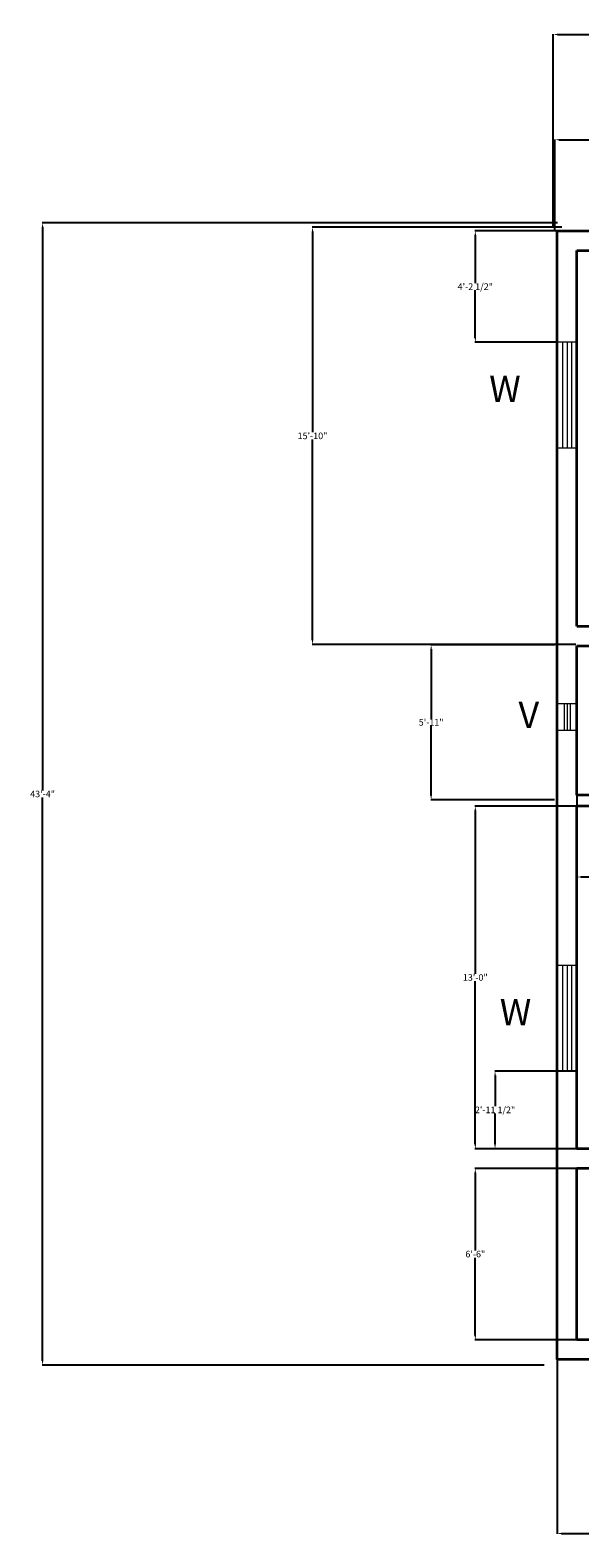
# Model space of a CAD drawing. Units: inches. Extents: x 751 to 1500, y 610 to 1297.
# Tile 1 of 4: x 751 to 1001, y 610 to 1297. Entities that reach past the tile are written whole.
import ezdxf

# ---------------------------------------------------------------- set-up
doc = ezdxf.new("R2010")
doc.units = ezdxf.units.IN
doc.header["$MEASUREMENT"] = 0
doc.layers.get('0').update_dxf_attribs({"color": 1})
for name, color, linetype, lineweight in [('A-ANNO-DIMS', 5, 'Continuous', 18), ('A-ANNO-TEXT', 7, 'Continuous', 18), ('wall', 6, 'Continuous', 35), ('windows', 70, 'Continuous', 18)]:
    doc.layers.add(name, color=color, linetype=linetype, lineweight=lineweight)
doc.styles.get("Standard").update_dxf_attribs({"font": 'arial.ttf'})
doc.dimstyles.get("Standard").update_dxf_attribs({"dimtxt": 3, "dimasz": 2, "dimexe": 0.18, "dimexo": 0.0625, "dimgap": 0.09, "dimtad": 0, "dimtih": 1, "dimtoh": 1, "dimdec": 0, "dimzin": 0, "dimdsep": 46, "dimlunit": 3, "dimtxsty": 'Standard', "dimcen": 0.09, "dimadec": 0, "dimazin": 0, "dimtfac": 1, "dimtdec": 0, "dimtofl": 0, "dimtmove": 0, "dimatfit": 3, "dimfxl": 1, "dimtolj": 1, "dimtzin": 0, "dimarcsym": 0})

# ---------------------------------------------------------------- blocks, each defined once
blk = doc.blocks.new('*D8')
at = {"layer": 'A-ANNO-DIMS', "color": 0, "lineweight": -2, "transparency": 16777216}
for p, q in [((989.16, 1207.18), (989.16, 1295.32)), ((991.16, 1295.14), (1215.8, 1295.14)), ((1450.93, 1295.14), (1226.29, 1295.14)), ((1452.93, 1205.96), (1452.93, 1295.32))]:
    blk.add_line(p, q, dxfattribs=at)
at = {"layer": 'A-ANNO-DIMS', "color": 0, "transparency": 16777216}
for points in [[(991.16, 1295.48), (991.16, 1294.81), (989.16, 1295.14)], [(1450.93, 1295.48), (1450.93, 1294.81), (1452.93, 1295.14)]]:
    blk.add_solid(points, dxfattribs=at)
at = {"layer": 'Defpoints', "color": 0, "transparency": 16777216}
for p in [(1452.93, 1295.14), (989.16, 1207.12), (1452.93, 1205.9)]:
    blk.add_point(p, dxfattribs=at)
at = {"layer": 'A-ANNO-DIMS', "color": 0, "transparency": 16777216, "insert": (1221.05, 1295.14), "char_height": 3, "attachment_point": 5}
blk.add_mtext('\\A1;38\'-8"', dxfattribs=at)
blk = doc.blocks.new('*D9')
at = {"layer": 'A-ANNO-DIMS', "color": 0, "lineweight": -2, "transparency": 16777216}
for p, q in [((989.97, 1205.95), (989.97, 1247.37)), ((991.97, 1247.19), (1077.79, 1247.19)), ((1173.82, 1247.19), (1088, 1247.19)), ((1175.82, 1205.95), (1175.82, 1247.37))]:
    blk.add_line(p, q, dxfattribs=at)
at = {"layer": 'A-ANNO-DIMS', "color": 0, "transparency": 16777216}
for points in [[(991.97, 1247.53), (991.97, 1246.86), (989.97, 1247.19)], [(1173.82, 1247.53), (1173.82, 1246.86), (1175.82, 1247.19)]]:
    blk.add_solid(points, dxfattribs=at)
at = {"layer": 'Defpoints', "color": 0, "transparency": 16777216}
for p in [(1175.82, 1247.19), (989.97, 1205.88), (1175.82, 1205.88)]:
    blk.add_point(p, dxfattribs=at)
at = {"layer": 'A-ANNO-DIMS', "color": 0, "transparency": 16777216, "insert": (1082.89, 1247.19), "char_height": 3, "attachment_point": 5}
blk.add_mtext('\\A1;15\'-6"', dxfattribs=at)
blk = doc.blocks.new('*D12')
at = {"layer": 'A-ANNO-DIMS', "color": 0, "lineweight": -2, "transparency": 16777216}
for p, q in [((991.09, 1209.39), (756.58, 1209.39)), ((756.76, 1207.39), (756.76, 950.89)), ((756.76, 691.14), (756.76, 947.64)), ((985.08, 689.14), (756.58, 689.14))]:
    blk.add_line(p, q, dxfattribs=at)
at = {"layer": 'A-ANNO-DIMS', "color": 0, "transparency": 16777216}
for points in [[(756.42, 1207.39), (757.09, 1207.39), (756.76, 1209.39)], [(756.42, 691.14), (757.09, 691.14), (756.76, 689.14)]]:
    blk.add_solid(points, dxfattribs=at)
at = {"layer": 'Defpoints', "color": 0, "transparency": 16777216}
for p in [(991.15, 1209.39), (756.76, 689.14), (985.14, 689.14)]:
    blk.add_point(p, dxfattribs=at)
at = {"layer": 'A-ANNO-DIMS', "color": 0, "transparency": 16777216, "insert": (756.76, 949.26), "char_height": 3, "attachment_point": 5}
blk.add_mtext('\\A1;43\'-4"', dxfattribs=at)
blk = doc.blocks.new('*D13')
at = {"layer": 'A-ANNO-DIMS', "color": 0, "lineweight": -2, "transparency": 16777216}
for p, q in [((993.09, 1207.39), (879.45, 1207.39)), ((879.63, 1205.39), (879.63, 1113.96)), ((879.63, 1019.29), (879.63, 1110.72)), ((999.43, 1017.29), (879.45, 1017.29))]:
    blk.add_line(p, q, dxfattribs=at)
at = {"layer": 'A-ANNO-DIMS', "color": 0, "transparency": 16777216}
for points in [[(879.3, 1205.39), (879.97, 1205.39), (879.63, 1207.39)], [(879.3, 1019.29), (879.97, 1019.29), (879.63, 1017.29)]]:
    blk.add_solid(points, dxfattribs=at)
at = {"layer": 'Defpoints', "color": 0, "transparency": 16777216}
for p in [(993.15, 1207.39), (879.63, 1017.29), (999.5, 1017.29)]:
    blk.add_point(p, dxfattribs=at)
at = {"layer": 'A-ANNO-DIMS', "color": 0, "transparency": 16777216, "insert": (879.63, 1112.34), "char_height": 3, "attachment_point": 5}
blk.add_mtext('\\A1;15\'-10"', dxfattribs=at)
blk = doc.blocks.new('*D14')
at = {"layer": 'A-ANNO-DIMS', "color": 0, "lineweight": -2, "transparency": 16777216}
for p, q in [((989.87, 1017.15), (933.44, 1017.15)), ((933.62, 1015.15), (933.62, 983.5)), ((933.62, 948.6), (933.62, 980.25)), ((989.8, 946.6), (933.44, 946.6))]:
    blk.add_line(p, q, dxfattribs=at)
at = {"layer": 'A-ANNO-DIMS', "color": 0, "transparency": 16777216}
for points in [[(933.29, 1015.15), (933.96, 1015.15), (933.62, 1017.15)], [(933.29, 948.6), (933.96, 948.6), (933.62, 946.6)]]:
    blk.add_solid(points, dxfattribs=at)
at = {"layer": 'Defpoints', "color": 0, "transparency": 16777216}
for p in [(989.93, 1017.15), (933.62, 946.6), (989.86, 946.6)]:
    blk.add_point(p, dxfattribs=at)
at = {"layer": 'A-ANNO-DIMS', "color": 0, "transparency": 16777216, "insert": (933.62, 981.87), "char_height": 3, "attachment_point": 5}
blk.add_mtext('\\A1;5\'-11"', dxfattribs=at)
blk = doc.blocks.new('WIN-48IN-PLAN')
for p, q in [((2.5, 48), (2.5, 0)), ((4.5, 48), (4.5, 0)), ((6.5, 48), (6.5, 0))]:
    blk.add_line(p, q)
blk.add_lwpolyline([(9, 48), (0, 48), (0, 0), (9, 0)], close=True)
blk = doc.blocks.new('VENT-12IN-PLAN')
for p, q in [((3.14, 12), (3.14, 0)), ((4.5, 12), (4.5, 0)), ((5.86, 12), (5.86, 0))]:
    blk.add_line(p, q)
blk.add_lwpolyline([(0, 0), (9, 0), (9, 12), (0, 12)], close=True)
blk = doc.blocks.new('*D47')
at = {"layer": 'A-ANNO-DIMS', "color": 0, "lineweight": -2, "transparency": 16777216}
for p, q in [((990.98, 691.63), (990.98, 612.26)), ((1176.98, 691.63), (1176.98, 612.26)), ((992.98, 612.44), (1078.88, 612.44)), ((1174.98, 612.44), (1089.08, 612.44))]:
    blk.add_line(p, q, dxfattribs=at)
at = {"layer": 'A-ANNO-DIMS', "color": 0, "transparency": 16777216}
for points in [[(992.98, 612.77), (992.98, 612.11), (990.98, 612.44)], [(1174.98, 612.77), (1174.98, 612.11), (1176.98, 612.44)]]:
    blk.add_solid(points, dxfattribs=at)
at = {"layer": 'Defpoints', "color": 0, "transparency": 16777216}
for p in [(990.98, 691.69), (1176.98, 691.69), (1176.98, 612.44)]:
    blk.add_point(p, dxfattribs=at)
at = {"layer": 'A-ANNO-DIMS', "color": 0, "transparency": 16777216, "insert": (1083.98, 612.44), "char_height": 3, "attachment_point": 5}
blk.add_mtext('\\A1;15\'-6"', dxfattribs=at)
blk = doc.blocks.new('*D49')
at = {"layer": 'A-ANNO-DIMS', "color": 0, "lineweight": -2, "transparency": 16777216}
for p, q in [((999.92, 778.69), (953.55, 778.69)), ((953.73, 776.69), (953.73, 741.31)), ((953.73, 702.69), (953.73, 738.07)), ((999.92, 700.69), (953.55, 700.69))]:
    blk.add_line(p, q, dxfattribs=at)
at = {"layer": 'A-ANNO-DIMS', "color": 0, "transparency": 16777216}
for points in [[(953.4, 776.69), (954.07, 776.69), (953.73, 778.69)], [(953.4, 702.69), (954.07, 702.69), (953.73, 700.69)]]:
    blk.add_solid(points, dxfattribs=at)
at = {"layer": 'Defpoints', "color": 0, "transparency": 16777216}
for p in [(953.73, 778.69), (999.98, 778.69), (999.98, 700.69)]:
    blk.add_point(p, dxfattribs=at)
at = {"layer": 'A-ANNO-DIMS', "color": 0, "transparency": 16777216, "insert": (953.73, 739.69), "char_height": 3, "attachment_point": 5}
blk.add_mtext('\\A1;6\'-6"', dxfattribs=at)
blk = doc.blocks.new('*D50')
at = {"layer": 'A-ANNO-DIMS', "color": 0, "lineweight": -2, "transparency": 16777216}
for p, q in [((999.92, 943.69), (953.55, 943.69)), ((953.73, 941.69), (953.73, 867.31)), ((953.73, 789.69), (953.73, 864.07)), ((999.92, 787.69), (953.55, 787.69))]:
    blk.add_line(p, q, dxfattribs=at)
at = {"layer": 'A-ANNO-DIMS', "color": 0, "transparency": 16777216}
for points in [[(953.4, 941.69), (954.07, 941.69), (953.73, 943.69)], [(953.4, 789.69), (954.07, 789.69), (953.73, 787.69)]]:
    blk.add_solid(points, dxfattribs=at)
at = {"layer": 'Defpoints', "color": 0, "transparency": 16777216}
for p in [(953.73, 943.69), (999.98, 943.69), (999.98, 787.69)]:
    blk.add_point(p, dxfattribs=at)
at = {"layer": 'A-ANNO-DIMS', "color": 0, "transparency": 16777216, "insert": (953.73, 865.69), "char_height": 3, "attachment_point": 5}
blk.add_mtext('\\A1;13\'-0"', dxfattribs=at)
blk = doc.blocks.new('*D54')
at = {"layer": 'A-ANNO-DIMS', "color": 0, "lineweight": -2, "transparency": 16777216}
for p, q in [((999.98, 948.63), (999.98, 911.26)), ((1083.98, 948.63), (1083.98, 911.26)), ((1001.98, 911.44), (1037.92, 911.44)), ((1081.98, 911.44), (1046.05, 911.44))]:
    blk.add_line(p, q, dxfattribs=at)
at = {"layer": 'A-ANNO-DIMS', "color": 0, "transparency": 16777216}
for points in [[(1001.98, 911.77), (1001.98, 911.11), (999.98, 911.44)], [(1081.98, 911.77), (1081.98, 911.11), (1083.98, 911.44)]]:
    blk.add_solid(points, dxfattribs=at)
at = {"layer": 'Defpoints', "color": 0, "transparency": 16777216}
for p in [(999.98, 948.69), (1083.98, 948.69), (999.98, 911.44)]:
    blk.add_point(p, dxfattribs=at)
at = {"layer": 'A-ANNO-DIMS', "color": 0, "transparency": 16777216, "insert": (1041.98, 911.44), "char_height": 3, "attachment_point": 5}
blk.add_mtext('\\A1;7\'-0"', dxfattribs=at)
blk = doc.blocks.new('*D63')
at = {"layer": 'A-ANNO-DIMS', "color": 0, "lineweight": -2, "transparency": 16777216}
for p, q in [((990.92, 1205.69), (953.55, 1205.69)), ((953.73, 1203.69), (953.73, 1181.96)), ((953.73, 1156.94), (953.73, 1178.68)), ((990.92, 1154.94), (953.55, 1154.94))]:
    blk.add_line(p, q, dxfattribs=at)
at = {"layer": 'A-ANNO-DIMS', "color": 0, "transparency": 16777216}
for points in [[(953.4, 1203.69), (954.07, 1203.69), (953.73, 1205.69)], [(953.4, 1156.94), (954.07, 1156.94), (953.73, 1154.94)]]:
    blk.add_solid(points, dxfattribs=at)
at = {"layer": 'Defpoints', "color": 0, "transparency": 16777216}
for p in [(953.73, 1205.69), (990.98, 1205.69), (990.98, 1154.94)]:
    blk.add_point(p, dxfattribs=at)
at = {"layer": 'A-ANNO-DIMS', "color": 0, "transparency": 16777216, "insert": (953.73, 1180.32), "char_height": 3, "attachment_point": 5}
blk.add_mtext('\\A1;4\'-2 1/2"', dxfattribs=at)
blk = doc.blocks.new('*D64')
at = {"layer": 'A-ANNO-DIMS', "color": 0, "lineweight": -2, "transparency": 16777216}
for p, q in [((999.92, 823.06), (962.55, 823.06)), ((962.73, 821.06), (962.73, 807.02)), ((962.73, 789.69), (962.73, 803.74)), ((999.92, 787.69), (962.55, 787.69))]:
    blk.add_line(p, q, dxfattribs=at)
at = {"layer": 'A-ANNO-DIMS', "color": 0, "transparency": 16777216}
for points in [[(962.4, 821.06), (963.07, 821.06), (962.73, 823.06)], [(962.4, 789.69), (963.07, 789.69), (962.73, 787.69)]]:
    blk.add_solid(points, dxfattribs=at)
at = {"layer": 'Defpoints', "color": 0, "transparency": 16777216}
for p in [(962.73, 823.06), (999.98, 823.06), (999.98, 787.69)]:
    blk.add_point(p, dxfattribs=at)
at = {"layer": 'A-ANNO-DIMS', "color": 0, "transparency": 16777216, "insert": (962.73, 805.38), "char_height": 3, "attachment_point": 5}
blk.add_mtext('\\A1;2\'-11 1/2"', dxfattribs=at)

msp = doc.modelspace()

# ---------------------------------------------------------------- linework, layer by layer
at = {"layer": 'wall'}
for p, q in [((990.98, 986.69), (990.98, 1205.69)), ((990.98, 1205.69), (1296.98, 1205.69)), ((999.98, 1196.69), (1171.98, 1196.69)), ((999.98, 1025.69), (999.98, 1196.69)), ((999.98, 1025.69), (1054.98, 1025.69)), ((999.98, 986.69), (999.98, 1016.69)), ((999.98, 1016.69), (1054.98, 1016.69)), ((990.98, 932.69), (990.98, 986.69)), ((999.98, 948.69), (999.98, 986.69)), ((1083.98, 948.69), (999.98, 948.69)), ((999.98, 932.69), (999.98, 943.69)), ((1171.98, 943.69), (999.98, 943.69)), ((990.98, 760.69), (990.98, 932.69)), ((999.98, 787.69), (999.98, 932.69)), ((1182.32, 787.69), (999.98, 787.69)), ((999.98, 760.69), (999.98, 778.69)), ((999.98, 700.69), (999.98, 778.69)), ((1182.32, 778.69), (999.98, 778.69)), ((990.98, 691.69), (990.98, 760.69)), ((1306.98, 700.69), (999.98, 700.69)), ((1171.98, 691.69), (990.98, 691.69))]:
    msp.add_line(p, q, dxfattribs=at)
at = {"layer": 'windows'}
for p, q in [((997.48, 871.06), (997.48, 823.06)), ((999.98, 871.06), (999.98, 823.06))]:
    msp.add_line(p, q, dxfattribs=at)
msp.add_lwpolyline([(999.98, 871.06), (990.98, 871.06), (990.98, 823.06), (999.98, 823.06)], close=True, dxfattribs=at)

# ---------------------------------------------------------------- block references
for name, p in [('WIN-48IN-PLAN', (990.98, 1106.94)), ('WIN-48IN-PLAN', (990.98, 1106.94)), ('VENT-12IN-PLAN', (990.98, 978.34)), ('WIN-48IN-PLAN', (990.98, 823.06))]:
    msp.add_blockref(name, p, dxfattribs=at)

# ---------------------------------------------------------------- texts
at = {"layer": 'A-ANNO-TEXT', "char_height": 12, "attachment_point": 1}
for s, width, insert in [('W', 41.6542, (960.05, 1139.72)), ('V', 67.5718, (973.37, 991.31)), ('W', 41.6542, (964.86, 855.94))]:
    msp.add_mtext_dynamic_manual_height_columns(s, width=width, gutter_width=1, heights=[0], dxfattribs=dict(at, insert=insert))

# ---------------------------------------------------------------- dimensions: what is measured, and where the dimension line sits
at = {"layer": 'A-ANNO-DIMS'}
for base, p1, p2, override, picture, middle in [((1452.93, 1295.14), (989.16, 1207.12), (1452.93, 1205.9), {"dimclrd": 0, "dimclre": 0, "dimclrt": 0}, '*D8', (1221.05, 1295.14)), ((1175.82, 1247.19), (989.97, 1205.88), (1175.82, 1205.88), {"dimclrd": 0, "dimclre": 0, "dimclrt": 0}, '*D9', (1082.89, 1247.19)), ((1176.98, 612.44), (990.98, 691.69), (1176.98, 691.69), {"dimdec": 1, "dimlfac": 1, "dimrnd": 0, "dimzin": 1, "dimdsep": 46, "dimlunit": 4, "dimfrac": 2}, '*D47', (1083.98, 612.44))]:
    dim = msp.add_linear_dim(base=base, p1=p1, p2=p2, dimstyle='Standard', override=override, dxfattribs=at)
    dim.commit()
    dim.dimension.update_dxf_attribs({"geometry": picture, "text_midpoint": middle})
for base, p1, p2, angle, override, picture, middle in [((756.76, 689.14), (991.15, 1209.39), (985.14, 689.14), 90, {"dimclrd": 0, "dimclre": 0, "dimclrt": 0}, '*D12', (756.76, 949.26)), ((879.63, 1017.29), (993.15, 1207.39), (999.5, 1017.29), 90, {"dimclrd": 0, "dimclre": 0, "dimclrt": 0}, '*D13', (879.63, 1112.34)), ((953.7324, 1205.6902), (990.9824, 1154.9446), (990.9824, 1205.6902), 90, {"dimdec": 1, "dimlfac": 1, "dimrnd": 0, "dimzin": 1, "dimdsep": 46, "dimlunit": 4, "dimfrac": 2}, '*D63', (953.7324, 1180.3174)), ((933.62, 946.6), (989.93, 1017.15), (989.86, 946.6), 90, {"dimclrd": 0, "dimclre": 0, "dimclrt": 0}, '*D14', (933.62, 981.87)), ((999.98, 911.44), (1083.98, 948.69), (999.98, 948.69), 180, {"dimdec": 1, "dimlfac": 1, "dimrnd": 0, "dimzin": 1, "dimdsep": 46, "dimlunit": 4, "dimfrac": 2}, '*D54', (1041.98, 911.44)), ((953.73, 943.69), (999.98, 787.69), (999.98, 943.69), 90, {"dimdec": 1, "dimlfac": 1, "dimrnd": 0, "dimzin": 1, "dimdsep": 46, "dimlunit": 4, "dimfrac": 2}, '*D50', (953.73, 865.69)), ((962.73, 823.06), (999.98, 787.69), (999.98, 823.06), 90, {"dimdec": 1, "dimlfac": 1, "dimrnd": 0, "dimzin": 1, "dimdsep": 46, "dimlunit": 4, "dimfrac": 2}, '*D64', (962.73, 805.38)), ((953.73, 778.69), (999.98, 700.69), (999.98, 778.69), 90, {"dimdec": 1, "dimlfac": 1, "dimrnd": 0, "dimzin": 1, "dimdsep": 46, "dimlunit": 4, "dimfrac": 2}, '*D49', (953.73, 739.69))]:
    dim = msp.add_linear_dim(base=base, p1=p1, p2=p2, angle=angle, dimstyle='Standard', override=override, dxfattribs=at)
    dim.commit()
    dim.dimension.update_dxf_attribs({"geometry": picture, "text_midpoint": middle})

doc.saveas('drawing.dxf')
